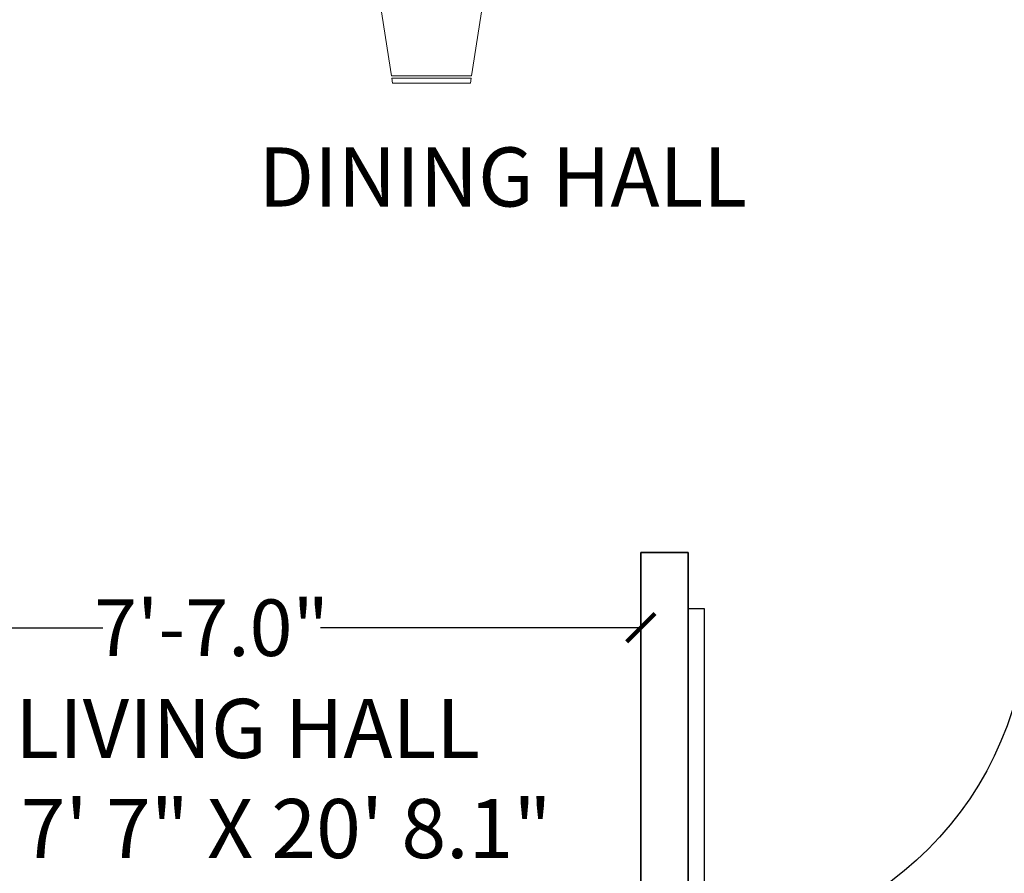
# Model space of a CAD drawing. Units: inches. Extents: x 844 to 2234, y 346 to 1084.
# Tile 90 of 93: x 1964 to 2069, y 737 to 828. Entities that reach past the tile are written whole.
import ezdxf

# ---------------------------------------------------------------- set-up
doc = ezdxf.new("R2010")
doc.units = ezdxf.units.IN
doc.header["$MEASUREMENT"] = 0
for name, color, linetype, lineweight in [('A-ANNO-DIMS', 2, 'Continuous', 18), ('A-AREA-IDEN', 7, 'Continuous', 18), ('A-WALL', 7, 'Continuous', 35), ('doors', 170, 'Continuous', 25), ('furniture', 8, 'Continuous', 18)]:
    doc.layers.add(name, color=color, linetype=linetype, lineweight=lineweight)
doc.styles.add('ATTR', font='romans.shx', dxfattribs={"width": 0.8, "height": 0.7})
doc.styles.get("Standard").update_dxf_attribs({"font": 'arial.ttf'})
doc.dimstyles.get("Standard").update_dxf_attribs({"dimtxt": 6, "dimasz": 3, "dimexe": 0.18, "dimexo": 0.0625, "dimgap": 0.09, "dimtad": 0, "dimtih": 1, "dimtoh": 1, "dimdec": 1, "dimzin": 0, "dimdsep": 46, "dimlunit": 3, "dimtxsty": 'Standard', "dimblk": 'ARCHTICK', "dimcen": 0.09, "dimadec": 0, "dimazin": 0, "dimtfac": 1, "dimtdec": 1, "dimtofl": 0, "dimtmove": 0, "dimatfit": 3, "dimfxl": 1, "dimtolj": 1, "dimtzin": 0, "dimarcsym": 0})

# ---------------------------------------------------------------- blocks, each defined once
blk = doc.blocks.new('*U2')
for p, q in [((0, 0), (0, -6)), ((36, 0), (36, -6))]:
    blk.add_line(p, q)
blk.add_lwpolyline([(0, 0), (0, 36), (1.75, 36), (1.75, 0)], close=True)
blk.add_arc((0, 0), 36, 0, 90)
blk = doc.blocks.new('DIN42X84')
for p, q in [((-34.772, 36.500609), (-37.0377, 21.999999)), ((-34.7681, 36.499999), (-18.2986, 36.499999)), ((-34.5377, 37.999999), (-34.6939, 37.000439)), ((-18.3793, 36.999999), (-34.6911, 36.999999)), ((-34.5377, 37.999999), (-18.5377, 37.999999)), ((-18.3814, 36.999659), (-18.5377, 37.999999)), ((-16.0377, 21.999999), (-18.3032, 36.499269)), ((-8.2343, 36.500609), (-10.5001, 21.999999)), ((-8.2305, 36.499999), (8.2391, 36.499999)), ((-8.0001, 37.999999), (-8.1562, 37.000439)), ((8.1584, 36.999999), (-8.1535, 36.999999)), ((-8.0001, 37.999999), (7.9999, 37.999999)), ((8.1562, 36.999659), (7.9999, 37.999999)), ((10.4999, 21.999999), (8.2344, 36.499269)), ((16.0376, 21.999999), (18.3031, 36.499269)), ((34.768, 36.499999), (18.2985, 36.499999)), ((18.3792, 36.999999), (34.691, 36.999999)), ((18.3813, 36.999659), (18.5376, 37.999999)), ((34.5376, 37.999999), (18.5376, 37.999999)), ((34.5376, 37.999999), (34.6938, 37.000439)), ((34.7719, 36.500609), (37.0376, 21.999999)), ((-43, 10.499989), (-57.4993, 8.234489)), ((43, 10.499989), (57.4992, 8.234489)), ((-57.9997, 8.156299), (-59, 7.999989)), ((-58, 8.158429), (-58, -8.153391)), ((-57.5, -8.230411), (-57.5, 8.239139)), ((57.5, -8.230411), (57.5, 8.239139)), ((57.9996, 8.156299), (59, 7.999989)), ((58, 8.158429), (58, -8.153391)), ((-59, -8.000011), (-59, 7.999989)), ((59, -8.000011), (59, 7.999989)), ((-59, -8.000011), (-58.0005, -8.156181)), ((59, -8.000011), (58.0004, -8.156181)), ((-57.5007, -8.234271), (-43, -10.500011)), ((57.5006, -8.234271), (43, -10.500011)), ((-42, -21.000001), (42, -21.000001)), ((-34.772, -36.50061), (-37.0377, -22.000001)), ((-16.0377, -22.000001), (-18.3032, -36.499267)), ((-8.2343, -36.50061), (-10.5001, -22.000001)), ((10.4999, -22.000001), (8.2344, -36.499267)), ((16.0376, -22.000001), (18.3031, -36.499267)), ((34.7719, -36.50061), (37.0376, -22.000001)), ((-34.7681, -36.499999), (-18.2986, -36.499999)), ((-34.5377, -37.999999), (-34.6939, -37.000442)), ((-18.3793, -36.999999), (-34.6911, -36.999999)), ((-34.5377, -37.999999), (-18.5377, -37.999999)), ((-18.3814, -36.999664), (-18.5377, -37.999999)), ((-8.2305, -36.499999), (8.2391, -36.499999)), ((-8.0001, -37.999999), (-8.1562, -37.000442)), ((8.1584, -36.999999), (-8.1535, -36.999999)), ((-8.0001, -37.999999), (7.9999, -37.999999)), ((8.1562, -36.999664), (7.9999, -37.999999)), ((34.768, -36.499999), (18.2985, -36.499999)), ((18.3792, -36.999999), (34.691, -36.999999)), ((18.3813, -36.999664), (18.5376, -37.999999)), ((34.5376, -37.999999), (18.5376, -37.999999)), ((34.5376, -37.999999), (34.6938, -37.000442))]:
    blk.add_line(p, q)
for points in [[(-42, -21.000001), (-42, 20.999989), (42, 20.999989), (42, -21.000001)], [(-42, 16.999989), (-40.5974, 16.672209), (-39.2569, 16.395939), (-37.9668, 16.166109), (-36.7153, 15.977689), (-35.4906, 15.825599), (-34.281, 15.704799), (-33.0745, 15.610229), (-31.8595, 15.536839), (-30.6267, 15.480229), (-29.3778, 15.438619), (-28.117, 15.410889), (-26.8486, 15.395929), (-25.5767, 15.392599), (-24.3058, 15.399809), (-23.0399, 15.416409), (-21.7833, 15.441309), (-20.5384, 15.473619), (-19.2994, 15.513549), (-18.0587, 15.561549), (-16.8087, 15.618049), (-15.5417, 15.683499), (-14.25, 15.758369), (-12.9261, 15.843079), (-11.5622, 15.938089), (-10.1541, 16.043559), (-8.7108, 16.158419), (-7.2445, 16.281349), (-5.7675, 16.410999), (-4.2923, 16.546019), (-2.8311, 16.685069), (-1.3963, 16.826809), (0, 16.969889), (1.3474, 17.113339), (2.6447, 17.257689), (3.8928, 17.403829), (5.0924, 17.552659), (6.2444, 17.705069), (7.3498, 17.861959), (8.4092, 18.024219), (9.4237, 18.192759), (10.3952, 18.367629), (11.3311, 18.545639), (12.2397, 18.722759), (13.1297, 18.894949), (14.0095, 19.058179), (14.8876, 19.208429), (15.7725, 19.341659), (16.6727, 19.453839), (17.5977, 19.541909), (18.5617, 19.606689), (19.5795, 19.649979), (20.6664, 19.673569), (21.8374, 19.679239), (23.1076, 19.668789), (24.492, 19.644009), (26.0058, 19.606689), (27.6589, 19.554579), (29.4413, 19.469229), (31.3377, 19.328169), (33.3331, 19.108889), (35.4121, 18.788919), (37.5598, 18.345779), (39.7608, 17.756959), (42, 16.999989)], [(42, 12.999999), (39.3635, 13.704689), (36.9303, 14.232849), (34.6868, 14.608169), (32.6195, 14.854319), (30.7149, 14.994989), (28.9596, 15.053859), (27.34, 15.054629), (25.8427, 15.020959), (24.4543, 14.972439), (23.1628, 14.912279), (21.9562, 14.839589), (20.8227, 14.753449), (19.7504, 14.652989), (18.7273, 14.537299), (17.7416, 14.405489), (16.7814, 14.256669), (15.8348, 14.090369), (14.8899, 13.907959), (13.9348, 13.711209), (12.9575, 13.501929), (11.9464, 13.281899), (10.8893, 13.052909), (9.7745, 12.816759), (8.59, 12.575229), (7.3261, 12.330049), (5.9815, 12.082619), (4.557, 11.834299), (3.0536, 11.586429), (1.472, 11.340349), (-0.187, 11.097409), (-1.9223, 10.858939), (-3.7333, 10.626289), (-5.6141, 10.400739), (-7.539, 10.183249), (-9.4776, 9.974709), (-11.3991, 9.776019), (-13.2731, 9.588079), (-15.0689, 9.411789), (-16.756, 9.248039), (-18.3038, 9.097709), (-19.6928, 8.961719), (-20.9483, 8.840959), (-22.1065, 8.736319), (-23.2037, 8.648689), (-24.2763, 8.578979), (-25.3606, 8.528079), (-26.4928, 8.496879), (-27.7094, 8.486279), (-29.0411, 8.496689), (-30.4965, 8.526549), (-32.0787, 8.573829), (-33.7908, 8.636479), (-35.6359, 8.712459), (-37.6171, 8.799739), (-39.7374, 8.896259), (-42, 8.999999)], [(-42, 0.999999), (-39.2567, 1.059739), (-36.6668, 1.127399), (-34.2177, 1.203389), (-31.897, 1.288099), (-29.6923, 1.381949), (-27.5912, 1.485329), (-25.5812, 1.598659), (-23.65, 1.722319), (-21.7874, 1.856519), (-19.9935, 2.000569), (-18.2704, 2.153579), (-16.6207, 2.314649), (-15.0465, 2.482879), (-13.5503, 2.657379), (-12.1344, 2.837259), (-10.8011, 3.021619), (-9.5514, 3.209479), (-8.3812, 3.399579), (-7.2848, 3.590579), (-6.2569, 3.781129), (-5.2918, 3.969889), (-4.384, 4.155509), (-3.5281, 4.336659), (-2.7184, 4.511979), (-1.9505, 4.680359), (-1.2233, 4.841579), (-0.5369, 4.995629), (0.1087, 5.142519), (0.7135, 5.282239), (1.2776, 5.414799), (1.8009, 5.540189), (2.2834, 5.658409), (2.7259, 5.769699), (3.1323, 5.875159), (3.5073, 5.976139), (3.8555, 6.073989), (4.1816, 6.170049), (4.4904, 6.265659), (4.7863, 6.362169), (5.0742, 6.460919), (5.3584, 6.563099), (5.6417, 6.669299), (5.9267, 6.779989), (6.216, 6.895609), (6.512, 7.016589), (6.8174, 7.143399), (7.1347, 7.276479), (7.4664, 7.416279), (7.8159, 7.563169), (8.1896, 7.717219), (8.5948, 7.878439), (9.0386, 8.046819), (9.5282, 8.222369), (10.071, 8.405079), (10.674, 8.594959), (11.3446, 8.791999), (12.0866, 8.995459), (12.8902, 9.201609), (13.7421, 9.405969), (14.6294, 9.604059), (15.5387, 9.791399), (16.4569, 9.963509), (17.3709, 10.115919), (18.2674, 10.244149), (19.1361, 10.344989), (19.9772, 10.420299), (20.7936, 10.473209), (21.5884, 10.506879), (22.3645, 10.524419), (23.1248, 10.528969), (23.8725, 10.523669), (24.6103, 10.511649), (25.3403, 10.495379), (26.0601, 10.474629), (26.7663, 10.448509), (27.4556, 10.416119), (28.1244, 10.376559), (28.7695, 10.328939), (29.3873, 10.272359), (29.9746, 10.205939), (30.5293, 10.129059), (31.0552, 10.042329), (31.5572, 9.946639), (32.0406, 9.842899), (32.5104, 9.731989), (32.9716, 9.614799), (33.4295, 9.492249), (33.8891, 9.365219), (34.3546, 9.234229), (34.8266, 9.098309), (35.3051, 8.956129), (35.7897, 8.806329), (36.2802, 8.647569), (36.7765, 8.478519), (37.2783, 8.297819), (37.7854, 8.104139), (38.2976, 7.894309), (38.8146, 7.657969), (39.3361, 7.382899), (39.8617, 7.056919), (40.3912, 6.667829), (40.9243, 6.203449), (41.4607, 5.651569), (42, 4.999999)], [(42, 0.999999), (35.1214, 2.295539), (25.1178, 2.983399), (7.9376, 2.295539), (0.3261, 1.149099), (-6.6329, -0.226611), (-18.3763, -2.978061), (-22.0733, -3.895201), (-27.5101, -4.583071), (-32.9468, -4.583071), (-35.339, -4.583071), (-38.3836, -4.353771), (-40.3408, -3.665921), (-42, -3.000001)], [(42, -3.000001), (38.9344, -2.781351), (35.8829, -2.650251), (32.8567, -2.595491), (29.8672, -2.605821), (26.9257, -2.670031), (24.0436, -2.776881), (21.2323, -2.915141), (18.5031, -3.073591), (15.8668, -3.242611), (13.3327, -3.419021), (10.9095, -3.601241), (8.6059, -3.787731), (6.4305, -3.976901), (4.3921, -4.167191), (2.4994, -4.357031), (0.7611, -4.544851), (-0.8196, -4.729651), (-2.2614, -4.912671), (-3.5885, -5.095681), (-4.8252, -5.280481), (-5.9956, -5.468861), (-7.1239, -5.662621), (-8.2344, -5.863551), (-9.3513, -6.073431), (-10.4925, -6.293091), (-11.6511, -6.519461), (-12.814, -6.748531), (-13.968, -6.976251), (-15.0999, -7.198591), (-16.1965, -7.411531), (-17.2447, -7.611041), (-18.2313, -7.793081), (-19.1472, -7.954521), (-19.9994, -8.095811), (-20.7989, -8.218291), (-21.5568, -8.323311), (-22.2841, -8.412201), (-22.9919, -8.486311), (-23.6912, -8.546991), (-24.393, -8.595581), (-25.1087, -8.632751), (-25.8513, -8.656491), (-26.6337, -8.664101), (-27.4693, -8.652901), (-28.3711, -8.620211), (-29.3523, -8.563341), (-30.4262, -8.479601), (-31.6057, -8.366301), (-32.8956, -8.222561), (-34.2657, -8.054761), (-35.6772, -7.871051), (-37.0913, -7.679611), (-38.4695, -7.488621), (-39.7728, -7.306241), (-40.9626, -7.140641), (-42, -7.000001)], [(-42, -15.000001), (-38.4722, -15.350691), (-35.3039, -15.623741), (-32.4544, -15.828971), (-29.8831, -15.976191), (-27.5493, -16.075201), (-25.4123, -16.135831), (-23.4313, -16.167881), (-21.5659, -16.181151), (-19.7812, -16.183881), (-18.0665, -16.177871), (-16.4173, -16.163351), (-14.8288, -16.140551), (-13.2964, -16.109691), (-11.8154, -16.070991), (-10.3811, -16.024671), (-8.9888, -15.970971), (-7.6345, -15.909991), (-6.3163, -15.841401), (-5.0329, -15.764751), (-3.7831, -15.679591), (-2.5656, -15.585471), (-1.3791, -15.481951), (-0.2223, -15.368571), (0.9061, -15.244901), (2.0079, -15.110631), (3.0876, -14.966051), (4.1503, -14.811631), (5.2011, -14.647801), (6.2451, -14.475011), (7.2875, -14.293721), (8.3332, -14.104361), (9.3874, -13.907391), (10.4544, -13.703711), (11.5349, -13.495991), (12.6291, -13.287381), (13.7368, -13.081011), (14.8581, -12.880011), (15.9931, -12.687521), (17.1416, -12.506671), (18.3037, -12.340601), (19.4778, -12.191771), (20.6562, -12.059961), (21.8295, -11.944271), (22.9884, -11.843811), (24.1234, -11.757681), (25.2254, -11.684981), (26.2848, -11.624831), (27.2925, -11.576311), (28.2412, -11.538551), (29.1325, -11.510631), (29.9703, -11.491671), (30.7584, -11.480781), (31.5007, -11.477041), (32.2009, -11.479581), (32.8628, -11.487491), (33.4904, -11.499881), (34.0874, -11.515741), (34.6576, -11.533621), (35.2049, -11.551941), (35.733, -11.569151), (36.2459, -11.583661), (36.7473, -11.593931), (37.2411, -11.598371), (37.7311, -11.595421), (38.2211, -11.583281), (38.7152, -11.559251), (39.2177, -11.520361), (39.7326, -11.463671), (40.2641, -11.386241), (40.8164, -11.285111), (41.3937, -11.157351), (42, -11.000001)]]:
    blk.add_lwpolyline(points)
for centre, start, end in [((-36.0377, 21.999999), 180, 270), ((-17.0377, 21.999999), 270, 0), ((-9.5001, 21.999999), 180, 270), ((9.4999, 21.999999), 270, 0), ((17.0376, 21.999999), 180, 270), ((36.0376, 21.999999), 270, 0), ((-43, 9.499989), 0.00000068, 90), ((43, 9.499989), 90, 180), ((-43, -9.500011), 270, 0.00000068), ((43, -9.500011), 180, 270), ((-36.0377, -22.000001), 90, 180), ((-17.0377, -22.000001), 0, 90), ((-9.5001, -22.000001), 90, 180), ((9.4999, -22.000001), 0, 90), ((17.0376, -22.000001), 90, 180), ((36.0376, -22.000001), 0, 90)]:
    blk.add_arc(centre, 1, start, end)
at = {"style": 'ATTR', "width": 0.8, "flags": 9}
blk.add_attdef('ESTCODE', (0, 0), '', height=0.7, dxfattribs=at)
blk = doc.blocks.new('_ArchTick')
at = {"color": 0, "linetype": 'ByBlock', "const_width": 0.15}
blk.add_lwpolyline([(-0.5, -0.5), (0.5, 0.5)], dxfattribs=at)
blk = doc.blocks.new('*D80')
at = {"layer": 'A-ANNO-DIMS', "color": 0, "lineweight": -2, "transparency": 16777216}
for p, q in [((1939.1, 763.54), (1939.1, 763.65)), ((1939.1, 763.47), (1973.06, 763.47)), ((2030.1, 763.47), (1996.13, 763.47)), ((2030.1, 763.54), (2030.1, 763.65))]:
    blk.add_line(p, q, dxfattribs=at)
at = {"layer": 'Defpoints', "color": 0, "transparency": 16777216}
for p in [(1939.1, 763.47), (1939.1, 763.47), (2030.1, 763.47)]:
    blk.add_point(p, dxfattribs=at)
at = {"layer": 'A-ANNO-DIMS', "color": 0, "lineweight": -2, "transparency": 16777216, "xscale": 3, "yscale": 3, "zscale": 3, "rotation": 180}
blk.add_blockref('_ArchTick', (1939.1, 763.47), dxfattribs=at)
at = {"layer": 'A-ANNO-DIMS', "color": 0, "lineweight": -2, "transparency": 16777216, "xscale": 3, "yscale": 3, "zscale": 3}
blk.add_blockref('_ArchTick', (2030.1, 763.47), dxfattribs=at)
at = {"layer": 'A-ANNO-DIMS', "color": 0, "transparency": 16777216, "insert": (1984.6, 763.47), "char_height": 6, "attachment_point": 5}
blk.add_mtext('\\A1;7\'-7.0"', dxfattribs=at)

msp = doc.modelspace()

# ---------------------------------------------------------------- linework, layer by layer
at = {"layer": 'A-WALL'}
for p, q in [((2035.1, 771.46), (2030.1, 771.46)), ((2030.1, 766.46), (2030.1, 771.46)), ((2035.1, 766.46), (2035.1, 771.46)), ((2030.1, 766.46), (2030.1, 629.46)), ((2035.1, 766.46), (2035.1, 634.46))]:
    msp.add_line(p, q, dxfattribs=at)

# ---------------------------------------------------------------- block references
at = {"layer": 'doors', "xscale": -1, "rotation": 180}
msp.add_blockref('*U2', (2035.1, 765.46), dxfattribs=at)
at = {"layer": 'furniture', "xscale": 0.5153672157522483, "yscale": 0.5153672157522483, "zscale": 0.5153672157522483, "rotation": 90}
msp.add_blockref('DIN42X84', (2007.91, 851.63), dxfattribs=at)

# ---------------------------------------------------------------- texts
at = {"layer": 'A-AREA-IDEN'}
for s, p in [('DINING HALL', (1989.58, 808.14)), ('  LIVING HALL', (1959.95, 749.66)), (' 7\' 7" X 20\' 8.1"', (1962.44, 739.04))]:
    msp.add_text(s, height=6.2688, dxfattribs=at).set_placement(p)

# ---------------------------------------------------------------- dimensions: what is measured, and where the dimension line sits
at = {"layer": 'A-ANNO-DIMS'}
dim = msp.add_linear_dim(base=(1939.1, 763.47), p1=(2030.1, 763.47), p2=(1939.1, 763.47), dimstyle='Standard', override={"dimclrd": 0, "dimclre": 0, "dimclrt": 0}, dxfattribs=at)
dim.commit()
dim.dimension.update_dxf_attribs({"geometry": '*D80', "text_midpoint": (1984.6, 763.47)})

doc.saveas('drawing.dxf')
